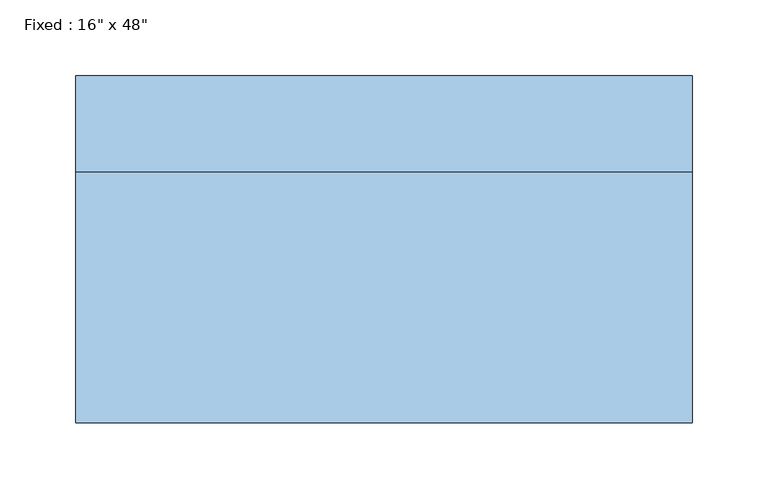
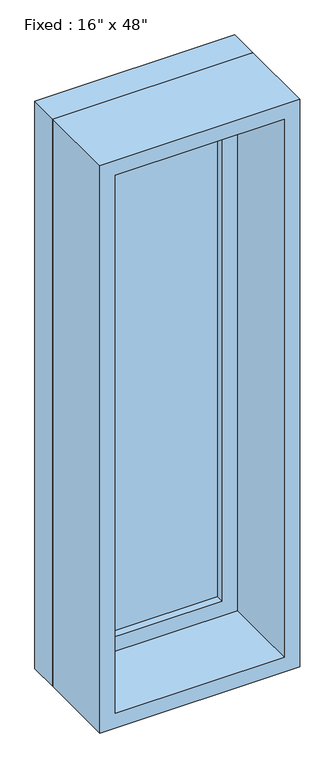
"""IFC4 building model written with IfcOpenShell, lengths in millimetres: window geometry."""

from ifc_helpers import new_model, si_unit, frame, origin, place, context, project, spatial, polyline, outline, extrude, source, transform, mapped, element, save


def window_cea7027f(model_context):
    return source(origin(), model_context, "Body", "SweptSolid", [
        extrude(outline(polyline([(101.6, 66.675), (-177.8, 66.675), (-177.8, 79.375), (101.6, 79.375), (101.6, 66.675)])), frame((0.0, 0.0, 977.9), z_axis=(0.0, 0.0, 1.0), x_axis=(1.0, 0.0, 0.0)), (0.0, 0.0, 1.0), 1092.2),
        extrude(outline(polyline([(2114.55, -222.25), (933.45, -222.25), (933.45, 146.05), (2114.55, 146.05), (2114.55, -222.25)]), holes=[polyline([(2070.1, -177.8), (2070.1, 101.6), (977.9, 101.6), (977.9, -177.8), (2070.1, -177.8)])]), frame((0.0, 50.8, 0.0), z_axis=(0.0, 1.0, 0.0), x_axis=(0.0, 0.0, 1.0)), (0.0, 0.0, 1.0), 44.45),
        extrude(outline(polyline([(2133.6, -241.3), (914.4, -241.3), (914.4, 165.1), (2133.6, 165.1), (2133.6, -241.3)]), holes=[polyline([(2101.85, -209.55), (2101.85, 133.35), (946.15, 133.35), (946.15, -209.55), (2101.85, -209.55)])]), frame((0.0, -114.3, 0.0), z_axis=(0.0, 1.0, 0.0), x_axis=(0.0, 0.0, 1.0)), (0.0, 0.0, 1.0), 165.1),
        extrude(outline(polyline([(2133.6, 165.1), (2133.6, -241.3), (914.4, -241.3), (914.4, 165.1), (2133.6, 165.1)]), holes=[polyline([(2114.55, 146.05), (933.45, 146.05), (933.45, -222.25), (2114.55, -222.25), (2114.55, 146.05)])]), frame((0.0, 50.8, 0.0), z_axis=(0.0, 1.0, 0.0), x_axis=(0.0, 0.0, 1.0)), (0.0, 0.0, 1.0), 63.5),
    ])


if __name__ == "__main__":
    model = new_model("IFC4")
    model_context = context("Model", 3, world=origin())
    ifc_project = project(units=[si_unit("LENGTHUNIT", "METRE", prefix="MILLI")], contexts=[model_context])
    site = spatial("IfcSite", under=ifc_project)
    building = spatial("IfcBuilding", under=site)
    placement = place(None, origin())
    window_shape = window_cea7027f(model_context)
    element("IfcWindow", 1, ObjectType="Fixed : 16\" x 48\"", at=placement, inside=building, context=model_context, shape_type="MappedRepresentation", body=[
        mapped(window_shape, transform((0.0, 0.0, 0.0), x_axis=(1.0, 0.0, 0.0), y_axis=(0.0, 1.0, 0.0), z_axis=(0.0, 0.0, 1.0))),
    ])
    save(model, "model.ifc")

# Revit data of these elements
# Type "Fixed : 16\" x 48\""
#   Type Mark = "5"
#   Construction Type Id = "GSP4R"
#   Assembly Code = "B2020100"
#   Analytic Construction = "1/8 in Pilkington single glazing"
#   Visual Light Transmittance = 0.9
#   Solar Heat Gain Coefficient = 0.78
#   Heat Transfer Coefficient (U) = 0.6496 BTU/(h·ft²·°F)
#   Height = 4' - 0"
#   Default Sill Height = 3' - 0"
#   Width = 1' - 4"
#   Window Inset = 0' - 0 3/4"
#   Define Thermal Properties by = 1
#   Define Thermal Properties by = 1
#   Glass Pane Material = Glass
#   Sash Material = Sash
#   Wall Closure = (empty or 0)
# Element 1 (IfcWindow, "Fixed : 16\" x 48\"")
#   Materials on its faces: "Sash", "Glass"
# Materials
#   "Glass": class "Glass", colour RGB 0 128 192, transparency 0.75, Description = "Soda Lime Glass", Cost = 0
#   "Sash": class "Wood", colour RGB 224 178 126, transparency 0, Cost = 0
